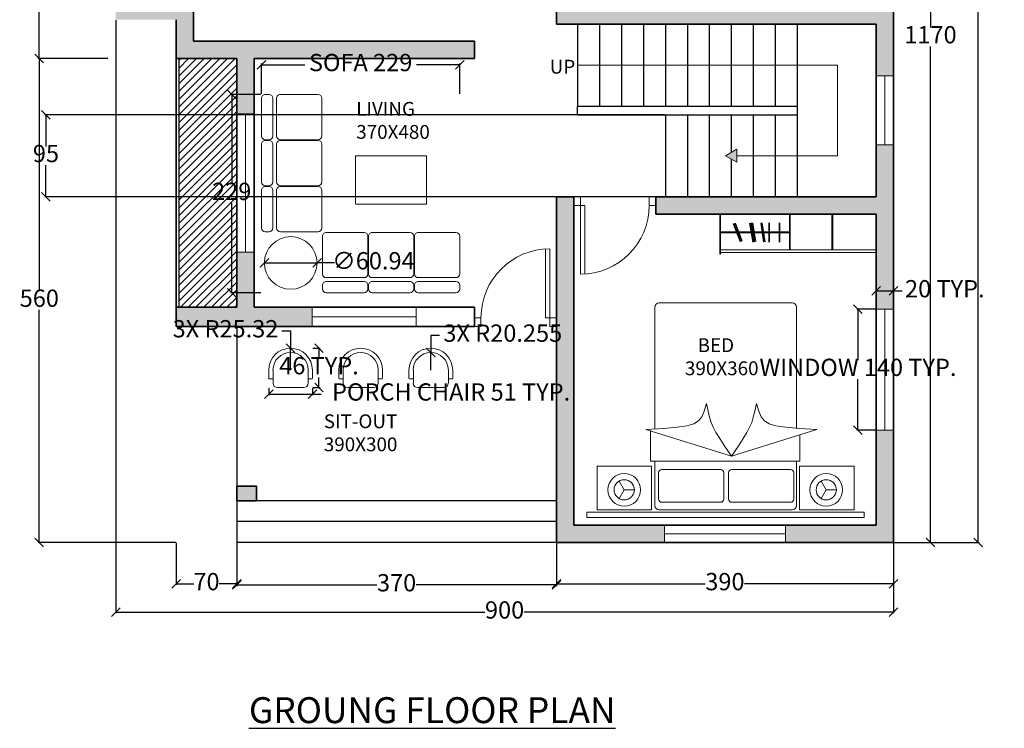
# Model space of a CAD drawing. Units: centimetres. Extents: x 2069 to 3209, y 376 to 1989.
# Tile 1 of 3: x 2069 to 3209, y 376 to 1196. Entities that reach past the tile are written whole.
import ezdxf

# ---------------------------------------------------------------- set-up
doc = ezdxf.new("R2010")
doc.units = ezdxf.units.CM
for name, color, linetype, lineweight in [('A-ANNO-DIMS', 2, 'Continuous', 18), ('A-ANNO-SYMB', 7, 'Continuous', 18), ('A-ANNO-TEXT', 7, 'Continuous', 25), ('A-AREA-IDEN', 7, 'Continuous', 25), ('A-COLS', 7, 'Continuous', 35), ('A-DOOR', 3, 'Continuous', 18), ('A-FLOR', 7, 'Continuous', 25), ('A-FLOR-CASE', 8, 'Continuous', 18), ('A-FLOR-PATT', 8, 'Continuous', 13), ('A-FLOR-STRS', 7, 'Continuous', 25), ('A-FURN', 8, 'Continuous', 18), ('A-GLAZ', 4, 'Continuous', 18), ('A-WALL', 7, 'Continuous', 35), ('A-WALL-PATT', 252, 'Continuous', 13)]:
    doc.layers.add(name, color=color, linetype=linetype, lineweight=lineweight)
doc.styles.get("Standard").update_dxf_attribs({"font": 'arial.ttf'})
doc.dimstyles.new('ISO-25', dxfattribs={"dimtxt": 20, "dimasz": 10, "dimexe": 1.25, "dimexo": 0.625, "dimtad": 0, "dimtih": 1, "dimtoh": 1, "dimtxsty": 'Standard', "dimblk": 'OBLIQUE', "dimcen": 6, "dimadec": 0, "dimazin": 0, "dimtfac": 1, "dimtmove": 0, "dimatfit": 3, "dimldrblk": 'OBLIQUE', "dimfxl": 1, "dimarcsym": 0})

# ---------------------------------------------------------------- blocks, each defined once
blk = doc.blocks.new('CAMMAT')
for p, q in [((1.2731, 0), (-1.2731, 0)), ((1.2731, 0), (1.2731, -0.05)), ((-1.2731, 0), (-1.2731, -0.05)), ((1.2731, -0.05), (-1.2731, -0.05)), ((-1.18, -0.07), (-1.18, -0.47)), ((-1.18, -0.07), (-0.68, -0.07)), ((-0.68, -0.07), (-0.68, -0.47)), ((0.61, -0.07), (-0.61, -0.07)), ((0.68, -0.07), (0.68, -0.47)), ((0.68, -0.07), (1.18, -0.07)), ((1.18, -0.07), (1.18, -0.47)), ((-0.931, -0.2541), (-0.9775, -0.1737)), ((-0.65, -0.11), (-0.65, -0.5169)), ((-0.6152, -0.1695), (-0.6152, -0.4095)), ((-0.0465, -0.1395), (-0.5852, -0.1395)), ((-0.0165, -0.1695), (-0.0165, -0.4095)), ((0.0274, -0.1695), (0.0274, -0.4095)), ((0.5962, -0.1395), (0.0574, -0.1395)), ((0.6262, -0.1695), (0.6262, -0.4095)), ((0.65, -0.11), (0.65, -0.5169)), ((0.9242, -0.2541), (0.8777, -0.1737)), ((-0.931, -0.2541), (-0.9775, -0.3346)), ((-0.931, -0.2541), (-0.8381, -0.2541)), ((0.9242, -0.2541), (0.8777, -0.3346)), ((0.9242, -0.2541), (1.0171, -0.2541)), ((-0.0465, -0.4395), (-0.5852, -0.4395)), ((0.5962, -0.4395), (0.0574, -0.4395)), ((-1.18, -0.47), (-0.68, -0.47)), ((-0.6904, -0.5169), (-0.6904, -0.8)), ((-0.6904, -0.5169), (0.6826, -0.5169)), ((0.68, -0.47), (1.18, -0.47)), ((0.6826, -0.5169), (0.6826, -0.7603)), ((0.0535, -0.5623), (-0.7312, -0.8093)), ((0.0535, -0.5623), (0.8382, -0.8093)), ((-0.65, -0.8139), (-0.65, -1.93)), ((0.65, -0.8204), (0.65, -1.93)), ((0.61, -1.97), (-0.61, -1.97))]:
    blk.add_line(p, q)
for points in [[(-0.1761, -1.0476), (-0.161, -0.9772), (-0.1474, -0.921), (-0.1326, -0.8732), (-0.1139, -0.8282), (-0.0886, -0.7803), (-0.0541, -0.7238), (-0.0076, -0.653), (0.0535, -0.5623)], [(0.2832, -1.0476), (0.2681, -0.9772), (0.2545, -0.921), (0.2396, -0.8732), (0.2209, -0.8282), (0.1957, -0.7803), (0.1611, -0.7238), (0.1147, -0.653), (0.0535, -0.5623)], [(-0.7312, -0.8093), (-0.5683, -0.8185), (-0.4451, -0.828), (-0.3552, -0.8406), (-0.2919, -0.8591), (-0.2489, -0.8862), (-0.2196, -0.9248), (-0.1975, -0.9777), (-0.1761, -1.0476)], [(0.8382, -0.8093), (0.6753, -0.8185), (0.5522, -0.828), (0.4622, -0.8406), (0.399, -0.8591), (0.356, -0.8862), (0.3267, -0.9248), (0.3046, -0.9777), (0.2832, -1.0476)]]:
    blk.add_lwpolyline(points)
for centre, radius in [((-0.931, -0.2541), 0.15), ((-0.931, -0.2541), 0.0929), ((0.9242, -0.2541), 0.15), ((0.9242, -0.2541), 0.0929)]:
    blk.add_circle(centre, radius)
for centre, radius, start, end in [((-0.61, -0.11), 0.04, 90, 180), ((0.61, -0.11), 0.04, 0, 90), ((-0.5852, -0.1695), 0.03, 90, 180), ((-0.0465, -0.1695), 0.03, 360, 90), ((0.0574, -0.1695), 0.03, 90, 180), ((0.5962, -0.1695), 0.03, 360, 90), ((-0.5852, -0.4095), 0.03, 180, 270), ((-0.0465, -0.4095), 0.03, 270, 360), ((0.0574, -0.4095), 0.03, 180, 270), ((0.5962, -0.4095), 0.03, 270, 360), ((-0.61, -1.93), 0.04, 180, 270), ((0.61, -1.93), 0.04, 270, 360)]:
    blk.add_arc(centre, radius, start, end)
blk = doc.blocks.new('A$C753D6792')
at = {"linetype": 'ByBlock'}
for p, q in [((50, 2630), (550, 2630)), ((660, 2630), (1160, 2630)), ((1270, 2630), (1770, 2630)), ((0, 2530), (0, 2580)), ((600, 2580), (600, 2530)), ((610, 2530), (610, 2580)), ((1210, 2580), (1210, 2530)), ((1220, 2530), (1220, 2580)), ((1820, 2580), (1820, 2530)), ((0, 1880), (0, 2380)), ((550, 2480), (50, 2480)), ((550, 2430), (50, 2430)), ((600, 2380), (600, 1880)), ((610, 1880), (610, 2380)), ((1160, 2480), (660, 2480)), ((1160, 2430), (660, 2430)), ((1210, 2380), (1210, 1880)), ((1220, 1880), (1220, 2380)), ((1770, 2480), (1270, 2480)), ((1770, 2430), (1270, 2430)), ((1820, 1880), (1820, 2380)), ((50, 1830), (427, 1830)), ((387, 1830), (550, 1830)), ((660, 1830), (1037, 1830)), ((997, 1830), (1160, 1830)), ((1270, 1830), (1647, 1830)), ((1607, 1830), (1770, 1830)), ((1830, 1770), (1830, 1393)), ((1880, 1820), (2380, 1820)), ((2430, 1270), (2430, 1770)), ((2480, 1270), (2480, 1770)), ((2530, 1820), (2580, 1820)), ((2630, 1770), (2630, 1270)), ((442, 815), (442, 1455)), ((442, 1455), (1372, 1455)), ((1382, 1455), (1382, 815)), ((1830, 1433), (1830, 1270)), ((2380, 1220), (1880, 1220)), ((1880, 1210), (2380, 1210)), ((2580, 1220), (2530, 1220)), ((2530, 1210), (2580, 1210)), ((1830, 1160), (1830, 783)), ((2430, 660), (2430, 1160)), ((2480, 660), (2480, 1160)), ((2630, 1160), (2630, 660)), ((1382, 815), (442, 815)), ((1830, 823), (1830, 660)), ((1830, 550), (1830, 173)), ((2380, 610), (1880, 610)), ((1880, 600), (2380, 600)), ((2430, 50), (2430, 550)), ((2480, 50), (2480, 550)), ((2580, 610), (2530, 610)), ((2530, 600), (2580, 600)), ((2630, 550), (2630, 50)), ((1830, 213), (1830, 50)), ((2380, 0), (1880, 0)), ((2580, 0), (2530, 0))]:
    blk.add_line(p, q, dxfattribs=at)
blk.add_circle((2242, 2235), 349, dxfattribs=at)
for centre, start, end in [((50, 2580), 90, 180), ((550, 2580), 0, 90), ((550, 2580), 0, 90), ((660, 2580), 90, 180), ((1160, 2580), 0, 90), ((1160, 2580), 0, 90), ((1270, 2580), 90, 180), ((1770, 2580), 0, 90), ((1770, 2580), 0, 90), ((50, 2530), 180, 270), ((550, 2530), 270, 0), ((550, 2530), 270, 0), ((660, 2530), 180, 270), ((1160, 2530), 270, 0), ((1160, 2530), 270, 0), ((1270, 2530), 180, 270), ((1770, 2530), 270, 0), ((1770, 2530), 270, 0), ((50, 2380), 90, 180), ((550, 2380), 0, 90), ((550, 2380), 0, 90), ((660, 2380), 90, 180), ((1160, 2380), 0, 90), ((1160, 2380), 0, 90), ((1270, 2380), 90, 180), ((1770, 2380), 0, 90), ((1770, 2380), 0, 90), ((50, 1880), 180, 270), ((550, 1880), 270, 0), ((660, 1880), 180, 270), ((1160, 1880), 270, 0), ((1270, 1880), 180, 270), ((1770, 1880), 270, 0), ((1880, 1770), 90, 180), ((2380, 1770), 0, 90), ((2530, 1770), 90, 180), ((2580, 1770), 0, 90), ((1880, 1270), 180, 270), ((1880, 1160), 90, 180), ((2380, 1270), 270, 0), ((2380, 1270), 270, 0), ((2380, 1160), 0, 90), ((2530, 1270), 180, 270), ((2530, 1270), 180, 270), ((2530, 1160), 90, 180), ((2580, 1270), 270, 0), ((2580, 1270), 270, 0), ((2580, 1160), 0, 90), ((1880, 660), 180, 270), ((2380, 660), 270, 0), ((2380, 660), 270, 0), ((2530, 660), 180, 270), ((2530, 660), 180, 270), ((2580, 660), 270, 0), ((2580, 660), 270, 0), ((1880, 550), 90, 180), ((2380, 550), 0, 90), ((2530, 550), 90, 180), ((2580, 550), 0, 90), ((1880, 50), 180, 270), ((2380, 50), 270, 0), ((2380, 50), 270, 0), ((2530, 50), 180, 270), ((2530, 50), 180, 270), ((2580, 50), 270, 0), ((2580, 50), 270, 0)]:
    blk.add_arc(centre, 50, start, end, dxfattribs=at)
blk = doc.blocks.new('_Oblique')
at = {"color": 0, "linetype": 'ByBlock', "lineweight": -2}
blk.add_line((-0.5, -0.5), (0.5, 0.5), dxfattribs=at)
blk = doc.blocks.new('*D16')
at = {"layer": 'A-ANNO-DIMS', "color": 0, "lineweight": -2, "transparency": 16777216}
for p, q in [((3081, 1761.2), (3124.6, 1761.2)), ((3123.3, 1761.2), (3123.3, 1187)), ((3123.3, 591.2), (3123.3, 1165.3)), ((3081, 591.2), (3124.6, 591.2))]:
    blk.add_line(p, q, dxfattribs=at)
at = {"layer": 'Defpoints', "color": 0, "transparency": 16777216}
for p in [(3080.4, 1761.2), (3080.4, 591.2), (3123.3, 591.2)]:
    blk.add_point(p, dxfattribs=at)
at = {"layer": 'A-ANNO-DIMS', "color": 0, "lineweight": -2, "transparency": 16777216, "xscale": 10, "yscale": 10, "zscale": 10}
for p, rotation in [((3123.3, 1761.2), 90), ((3123.3, 591.2), 270)]:
    blk.add_blockref('_Oblique', p, dxfattribs=dict(at, rotation=rotation))
at = {"layer": 'A-ANNO-DIMS', "color": 0, "transparency": 16777216, "insert": (3123.3, 1176.2), "char_height": 20, "attachment_point": 5}
blk.add_mtext('1170', dxfattribs=at)
blk = doc.blocks.new('*D17')
at = {"layer": 'A-ANNO-DIMS', "color": 0, "lineweight": -2, "transparency": 16777216}
for p, q in [((2690.4, 590.6), (2690.4, 541.9)), ((3080.4, 590.6), (3080.4, 541.9)), ((2690.4, 543.2), (2862.7, 543.2)), ((3080.4, 543.2), (2908.1, 543.2))]:
    blk.add_line(p, q, dxfattribs=at)
at = {"layer": 'Defpoints', "color": 0, "transparency": 16777216}
for p in [(2690.4, 591.2), (3080.4, 591.2), (2690.4, 543.2)]:
    blk.add_point(p, dxfattribs=at)
at = {"layer": 'A-ANNO-DIMS', "color": 0, "lineweight": -2, "transparency": 16777216, "xscale": 10, "yscale": 10, "zscale": 10, "rotation": 180}
blk.add_blockref('_Oblique', (2690.4, 543.2), dxfattribs=at)
at = {"layer": 'A-ANNO-DIMS', "color": 0, "lineweight": -2, "transparency": 16777216, "xscale": 10, "yscale": 10, "zscale": 10}
blk.add_blockref('_Oblique', (3080.4, 543.2), dxfattribs=at)
at = {"layer": 'A-ANNO-DIMS', "color": 0, "transparency": 16777216, "insert": (2885.4, 543.2), "char_height": 20, "attachment_point": 5}
blk.add_mtext('390', dxfattribs=at)
blk = doc.blocks.new('*D18')
at = {"layer": 'A-ANNO-DIMS', "color": 0, "lineweight": -2, "transparency": 16777216}
for p, q in [((2320.4, 590.6), (2320.4, 540.7)), ((2690.4, 590.6), (2690.4, 540.7)), ((2320.4, 541.9), (2482.7, 541.9)), ((2690.4, 541.9), (2528.1, 541.9))]:
    blk.add_line(p, q, dxfattribs=at)
at = {"layer": 'Defpoints', "color": 0, "transparency": 16777216}
for p in [(2320.4, 591.2), (2690.4, 591.2), (2320.4, 541.9)]:
    blk.add_point(p, dxfattribs=at)
at = {"layer": 'A-ANNO-DIMS', "color": 0, "lineweight": -2, "transparency": 16777216, "xscale": 10, "yscale": 10, "zscale": 10, "rotation": 180}
blk.add_blockref('_Oblique', (2320.4, 541.9), dxfattribs=at)
at = {"layer": 'A-ANNO-DIMS', "color": 0, "lineweight": -2, "transparency": 16777216, "xscale": 10, "yscale": 10, "zscale": 10}
blk.add_blockref('_Oblique', (2690.4, 541.9), dxfattribs=at)
at = {"layer": 'A-ANNO-DIMS', "color": 0, "transparency": 16777216, "insert": (2505.4, 541.9), "char_height": 20, "attachment_point": 5}
blk.add_mtext('370', dxfattribs=at)
blk = doc.blocks.new('*D19')
at = {"layer": 'A-ANNO-DIMS', "color": 0, "lineweight": -2, "transparency": 16777216}
for p, q in [((2250.4, 590.6), (2250.4, 541.9)), ((2320.4, 590.6), (2320.4, 541.9)), ((2250.4, 543.2), (2270.6, 543.2)), ((2320.4, 543.2), (2300.2, 543.2))]:
    blk.add_line(p, q, dxfattribs=at)
at = {"layer": 'Defpoints', "color": 0, "transparency": 16777216}
for p in [(2250.4, 591.2), (2320.4, 591.2), (2320.4, 543.2)]:
    blk.add_point(p, dxfattribs=at)
at = {"layer": 'A-ANNO-DIMS', "color": 0, "lineweight": -2, "transparency": 16777216, "xscale": 10, "yscale": 10, "zscale": 10, "rotation": 180}
blk.add_blockref('_Oblique', (2250.4, 543.2), dxfattribs=at)
at = {"layer": 'A-ANNO-DIMS', "color": 0, "lineweight": -2, "transparency": 16777216, "xscale": 10, "yscale": 10, "zscale": 10}
blk.add_blockref('_Oblique', (2320.4, 543.2), dxfattribs=at)
at = {"layer": 'A-ANNO-DIMS', "color": 0, "transparency": 16777216, "insert": (2285.4, 543.2), "char_height": 20, "attachment_point": 5}
blk.add_mtext('70', dxfattribs=at)
blk = doc.blocks.new('*D21')
at = {"layer": 'A-ANNO-DIMS', "color": 0, "lineweight": -2, "transparency": 16777216}
for p, q in [((2170.2, 1521.2), (2090.7, 1521.2)), ((2091.9, 1521.2), (2091.9, 1347)), ((2091.9, 1151.2), (2091.9, 1325.3)), ((2171.1, 1151.2), (2090.7, 1151.2))]:
    blk.add_line(p, q, dxfattribs=at)
at = {"layer": 'Defpoints', "color": 0, "transparency": 16777216}
for p in [(2170.8, 1521.2), (2091.9, 1151.2), (2171.7, 1151.2)]:
    blk.add_point(p, dxfattribs=at)
at = {"layer": 'A-ANNO-DIMS', "color": 0, "lineweight": -2, "transparency": 16777216, "xscale": 10, "yscale": 10, "zscale": 10}
for p, rotation in [((2091.9, 1521.2), 90), ((2091.9, 1151.2), 270)]:
    blk.add_blockref('_Oblique', p, dxfattribs=dict(at, rotation=rotation))
at = {"layer": 'A-ANNO-DIMS', "color": 0, "transparency": 16777216, "insert": (2091.9, 1336.2), "char_height": 20, "attachment_point": 5}
blk.add_mtext('370', dxfattribs=at)
blk = doc.blocks.new('*D22')
at = {"layer": 'A-ANNO-DIMS', "color": 0, "lineweight": -2, "transparency": 16777216}
for p, q in [((2169.6, 1151.2), (2090.7, 1151.2)), ((2091.9, 1151.2), (2091.9, 882)), ((2091.9, 591.2), (2091.9, 860.3)), ((2249.8, 591.2), (2090.7, 591.2))]:
    blk.add_line(p, q, dxfattribs=at)
at = {"layer": 'Defpoints', "color": 0, "transparency": 16777216}
for p in [(2170.2, 1151.2), (2091.9, 591.2), (2250.4, 591.2)]:
    blk.add_point(p, dxfattribs=at)
at = {"layer": 'A-ANNO-DIMS', "color": 0, "lineweight": -2, "transparency": 16777216, "xscale": 10, "yscale": 10, "zscale": 10}
for p, rotation in [((2091.9, 1151.2), 90), ((2091.9, 591.2), 270)]:
    blk.add_blockref('_Oblique', p, dxfattribs=dict(at, rotation=rotation))
at = {"layer": 'A-ANNO-DIMS', "color": 0, "transparency": 16777216, "insert": (2091.9, 871.2), "char_height": 20, "attachment_point": 5}
blk.add_mtext('560', dxfattribs=at)
blk = doc.blocks.new('CHAIR-SITOUT')
for p, q in [((0, 11.1), (0, 20.3)), ((5.1, 20.3), (5.1, 5.1)), ((45.6, 5.1), (45.6, 20.3)), ((50.6, 11.1), (50.6, 20.3)), ((1, 10.1), (5.1, 10.1)), ((10.1, 0), (40.5, 0)), ((45.6, 10.1), (49.6, 10.1))]:
    blk.add_line(p, q)
for centre, radius, start, end in [((25.3, 20.3), 25.3, 0, 180), ((25.3, 20.3), 20.3, 0.0001, 179.9999), ((1, 11.1), 1.01, 180, 270), ((10.1, 5.1), 5.06, 180, 270), ((40.5, 5.1), 5.06, 270, 0), ((49.6, 11.1), 1.01, 270, 0)]:
    blk.add_arc(centre, radius, start, end)
blk = doc.blocks.new('WIN-1400')
for p, q in [((0, 140), (20, 140)), ((10, 0), (10, 140)), ((0, 0), (20, 0))]:
    blk.add_line(p, q)
blk = doc.blocks.new('DOOR-SINGLE-950')
for p, q in [((82.3, 89.4), (82.3, 10)), ((87.3, 89.6), (87.3, 10)), ((0, 10), (7.7, 10)), ((7.7, 10), (7.7, 0)), ((82.3, 10), (87.3, 10)), ((95, 10), (87.3, 10)), ((87.3, 10), (87.3, 0)), ((7.7, 0), (0, 0)), ((87.3, 0), (95, 0))]:
    blk.add_line(p, q)
blk.add_arc((87.3, 10), 79.6, 90, 180)
blk = doc.blocks.new('*D32')
at = {"layer": 'A-ANNO-DIMS', "color": 0, "lineweight": -2, "transparency": 16777216}
for p, q in [((2357.4, 769.7), (2357.4, 761.4)), ((2408, 769.7), (2408, 761.4)), ((2357.4, 762.7), (2408, 762.7)), ((2408, 762.7), (2418, 762.7))]:
    blk.add_line(p, q, dxfattribs=at)
at = {"layer": 'Defpoints', "color": 0, "transparency": 16777216}
for p in [(2357.4, 770.3), (2408, 770.3), (2408, 762.7)]:
    blk.add_point(p, dxfattribs=at)
at = {"layer": 'A-ANNO-DIMS', "color": 0, "lineweight": -2, "transparency": 16777216, "xscale": 10, "yscale": 10, "zscale": 10, "rotation": 180}
blk.add_blockref('_Oblique', (2357.4, 762.7), dxfattribs=at)
at = {"layer": 'A-ANNO-DIMS', "color": 0, "lineweight": -2, "transparency": 16777216, "xscale": 10, "yscale": 10, "zscale": 10}
blk.add_blockref('_Oblique', (2408, 762.7), dxfattribs=at)
at = {"layer": 'A-ANNO-DIMS', "color": 0, "transparency": 16777216, "insert": (2568.5, 762.7), "char_height": 20, "attachment_point": 5}
blk.add_mtext('PORCH CHAIR 51 TYP.', dxfattribs=at)
blk = doc.blocks.new('*D33')
at = {"layer": 'A-ANNO-DIMS', "color": 0, "lineweight": -2, "transparency": 16777216}
for p, q in [((2408.6, 815.9), (2416.8, 815.9)), ((2415.6, 815.9), (2415.6, 803.9)), ((2415.6, 770.3), (2415.6, 782.2)), ((2408.6, 770.3), (2416.8, 770.3))]:
    blk.add_line(p, q, dxfattribs=at)
at = {"layer": 'Defpoints', "color": 0, "transparency": 16777216}
for p in [(2408, 815.9), (2415.6, 815.9), (2408, 770.3)]:
    blk.add_point(p, dxfattribs=at)
at = {"layer": 'A-ANNO-DIMS', "color": 0, "lineweight": -2, "transparency": 16777216, "xscale": 10, "yscale": 10, "zscale": 10}
for p, rotation in [((2415.6, 815.9), 90), ((2415.6, 770.3), 270)]:
    blk.add_blockref('_Oblique', p, dxfattribs=dict(at, rotation=rotation))
at = {"layer": 'A-ANNO-DIMS', "color": 0, "transparency": 16777216, "insert": (2415.6, 793.1), "char_height": 20, "attachment_point": 5}
blk.add_mtext('46 TYP.', dxfattribs=at)
blk = doc.blocks.new('*D34')
at = {"layer": 'A-ANNO-DIMS', "color": 0, "lineweight": -2, "transparency": 16777216}
for p, q in [((3059.8, 861.2), (3038.1, 861.2)), ((3039.4, 861.2), (3039.4, 802.2)), ((3039.4, 721.2), (3039.4, 780.2)), ((3059.8, 721.2), (3038.1, 721.2))]:
    blk.add_line(p, q, dxfattribs=at)
at = {"layer": 'Defpoints', "color": 0, "transparency": 16777216}
for p in [(3039.4, 861.2), (3060.4, 861.2), (3060.4, 721.2)]:
    blk.add_point(p, dxfattribs=at)
at = {"layer": 'A-ANNO-DIMS', "color": 0, "lineweight": -2, "transparency": 16777216, "xscale": 10, "yscale": 10, "zscale": 10}
for p, rotation in [((3039.4, 861.2), 90), ((3039.4, 721.2), 270)]:
    blk.add_blockref('_Oblique', p, dxfattribs=dict(at, rotation=rotation))
at = {"layer": 'A-ANNO-DIMS', "color": 0, "transparency": 16777216, "insert": (3039.4, 791.2), "char_height": 20, "attachment_point": 5}
blk.add_mtext('WINDOW 140 TYP.', dxfattribs=at)
blk = doc.blocks.new('*D35')
at = {"layer": 'A-ANNO-DIMS', "color": 0, "lineweight": -2, "transparency": 16777216}
for p, q in [((3060.4, 861.8), (3060.4, 883.4)), ((3060.4, 882.2), (3080.4, 882.2)), ((3080.4, 861.8), (3080.4, 883.4)), ((3080.4, 882.2), (3090.4, 882.2))]:
    blk.add_line(p, q, dxfattribs=at)
at = {"layer": 'Defpoints', "color": 0, "transparency": 16777216}
for p in [(3080.4, 882.2), (3060.4, 861.2), (3080.4, 861.2)]:
    blk.add_point(p, dxfattribs=at)
at = {"layer": 'A-ANNO-DIMS', "color": 0, "lineweight": -2, "transparency": 16777216, "xscale": 10, "yscale": 10, "zscale": 10, "rotation": 180}
blk.add_blockref('_Oblique', (3060.4, 882.2), dxfattribs=at)
at = {"layer": 'A-ANNO-DIMS', "color": 0, "lineweight": -2, "transparency": 16777216, "xscale": 10, "yscale": 10, "zscale": 10}
blk.add_blockref('_Oblique', (3080.4, 882.2), dxfattribs=at)
at = {"layer": 'A-ANNO-DIMS', "color": 0, "transparency": 16777216, "insert": (3139.9, 882.2), "char_height": 20, "attachment_point": 5}
blk.add_mtext('20 TYP.', dxfattribs=at)
blk = doc.blocks.new('*D44')
at = {"layer": 'A-ANNO-DIMS', "color": 0, "lineweight": -2, "transparency": 16777216}
for p, q in [((2349.1, 1110.2), (2349.1, 1145.3)), ((2349.1, 1144), (2399.2, 1144)), ((2578.5, 1144), (2528.4, 1144)), ((2578.5, 1110.2), (2578.5, 1145.3))]:
    blk.add_line(p, q, dxfattribs=at)
at = {"layer": 'Defpoints', "color": 0, "transparency": 16777216}
for p in [(2349.1, 1144), (2349.1, 1109.6), (2578.5, 1109.6)]:
    blk.add_point(p, dxfattribs=at)
at = {"layer": 'A-ANNO-DIMS', "color": 0, "lineweight": -2, "transparency": 16777216, "xscale": 10, "yscale": 10, "zscale": 10, "rotation": 180}
blk.add_blockref('_Oblique', (2349.1, 1144), dxfattribs=at)
at = {"layer": 'A-ANNO-DIMS', "color": 0, "lineweight": -2, "transparency": 16777216, "xscale": 10, "yscale": 10, "zscale": 10}
blk.add_blockref('_Oblique', (2578.5, 1144), dxfattribs=at)
at = {"layer": 'A-ANNO-DIMS', "color": 0, "transparency": 16777216, "insert": (2463.8, 1144), "char_height": 20, "attachment_point": 5}
blk.add_mtext('SOFA 229', dxfattribs=at)
blk = doc.blocks.new('*D45')
at = {"layer": 'A-ANNO-DIMS', "color": 0, "lineweight": -2, "transparency": 16777216}
for p, q in [((2348.4, 1109.6), (2313.4, 1109.6)), ((2314.6, 1109.6), (2314.6, 1005.7)), ((2314.6, 880.1), (2314.6, 984)), ((2348.4, 880.1), (2313.4, 880.1))]:
    blk.add_line(p, q, dxfattribs=at)
at = {"layer": 'Defpoints', "color": 0, "transparency": 16777216}
for p in [(2349.1, 1109.6), (2314.6, 880.1), (2349.1, 880.1)]:
    blk.add_point(p, dxfattribs=at)
at = {"layer": 'A-ANNO-DIMS', "color": 0, "lineweight": -2, "transparency": 16777216, "xscale": 10, "yscale": 10, "zscale": 10}
for p, rotation in [((2314.6, 1109.6), 90), ((2314.6, 880.1), 270)]:
    blk.add_blockref('_Oblique', p, dxfattribs=dict(at, rotation=rotation))
at = {"layer": 'A-ANNO-DIMS', "color": 0, "transparency": 16777216, "insert": (2314.6, 994.9), "char_height": 20, "attachment_point": 5}
blk.add_mtext('229', dxfattribs=at)
blk = doc.blocks.new('*D46')
at = {"layer": 'A-ANNO-DIMS', "color": 0, "lineweight": -2, "transparency": 16777216}
for p, q in [((2180.4, 1195.6), (2180.4, 509.1)), ((3080.4, 590.6), (3080.4, 509.1)), ((2180.4, 510.4), (2607.7, 510.4)), ((3080.4, 510.4), (2653.1, 510.4))]:
    blk.add_line(p, q, dxfattribs=at)
at = {"layer": 'Defpoints', "color": 0, "transparency": 16777216}
for p in [(2180.4, 1196.2), (3080.4, 591.2), (3080.4, 510.4)]:
    blk.add_point(p, dxfattribs=at)
at = {"layer": 'A-ANNO-DIMS', "color": 0, "lineweight": -2, "transparency": 16777216, "xscale": 10, "yscale": 10, "zscale": 10, "rotation": 180}
blk.add_blockref('_Oblique', (2180.4, 510.4), dxfattribs=at)
at = {"layer": 'A-ANNO-DIMS', "color": 0, "lineweight": -2, "transparency": 16777216, "xscale": 10, "yscale": 10, "zscale": 10}
blk.add_blockref('_Oblique', (3080.4, 510.4), dxfattribs=at)
at = {"layer": 'A-ANNO-DIMS', "color": 0, "transparency": 16777216, "insert": (2630.4, 510.4), "char_height": 20, "attachment_point": 5}
blk.add_mtext('900', dxfattribs=at)
blk = doc.blocks.new('*D47')
at = {"layer": 'A-ANNO-DIMS', "color": 0, "lineweight": -2, "transparency": 16777216}
for p, q in [((2711, 1941.2), (3179.7, 1941.2)), ((3178.5, 1941.2), (3178.5, 1277)), ((3178.5, 591.2), (3178.5, 1255.3)), ((3081, 591.2), (3179.7, 591.2))]:
    blk.add_line(p, q, dxfattribs=at)
at = {"layer": 'Defpoints', "color": 0, "transparency": 16777216}
for p in [(2710.4, 1941.2), (3080.4, 591.2), (3178.5, 591.2)]:
    blk.add_point(p, dxfattribs=at)
at = {"layer": 'A-ANNO-DIMS', "color": 0, "lineweight": -2, "transparency": 16777216, "xscale": 10, "yscale": 10, "zscale": 10}
for p, rotation in [((3178.5, 1941.2), 90), ((3178.5, 591.2), 270)]:
    blk.add_blockref('_Oblique', p, dxfattribs=dict(at, rotation=rotation))
at = {"layer": 'A-ANNO-DIMS', "color": 0, "transparency": 16777216, "insert": (3178.5, 1266.2), "char_height": 20, "attachment_point": 5}
blk.add_mtext('1350', dxfattribs=at)
blk = doc.blocks.new('*D48')
at = {"layer": 'A-ANNO-DIMS', "color": 0, "lineweight": -2, "transparency": 16777216}
for p, q in [((2815.9, 1086.2), (2098.3, 1086.2)), ((2099.6, 1086.2), (2099.6, 1049.5)), ((2099.6, 991.2), (2099.6, 1027.8)), ((2815.9, 991.2), (2098.3, 991.2))]:
    blk.add_line(p, q, dxfattribs=at)
at = {"layer": 'Defpoints', "color": 0, "transparency": 16777216}
for p in [(2099.6, 1086.2), (2816.5, 1086.2), (2816.5, 991.2)]:
    blk.add_point(p, dxfattribs=at)
at = {"layer": 'A-ANNO-DIMS', "color": 0, "lineweight": -2, "transparency": 16777216, "xscale": 10, "yscale": 10, "zscale": 10}
for p, rotation in [((2099.6, 1086.2), 90), ((2099.6, 991.2), 270)]:
    blk.add_blockref('_Oblique', p, dxfattribs=dict(at, rotation=rotation))
at = {"layer": 'A-ANNO-DIMS', "color": 0, "transparency": 16777216, "insert": (2099.6, 1038.7), "char_height": 20, "attachment_point": 5}
blk.add_mtext('95', dxfattribs=at)
blk = doc.blocks.new('*D49')
at = {"layer": 'A-ANNO-DIMS', "color": 0, "lineweight": -2, "transparency": 16777216}
for p in [(2352.4, 914.6), (2433.4, 914.6)]:
    blk.add_line(p, (2413.4, 914.6), dxfattribs=at)
at = {"layer": 'Defpoints', "color": 0, "transparency": 16777216}
for p in [(2352.4, 914.6), (2413.4, 914.6)]:
    blk.add_point(p, dxfattribs=at)
at = {"layer": 'A-ANNO-DIMS', "color": 0, "lineweight": -2, "transparency": 16777216, "xscale": 10, "yscale": 10, "zscale": 10}
for p, rotation in [((2352.4, 914.6), 0.0003591282010973), ((2413.4, 914.6), 180.0003591282011)]:
    blk.add_blockref('_Oblique', p, dxfattribs=dict(at, rotation=rotation))
at = {"layer": 'A-ANNO-DIMS', "color": 0, "transparency": 16777216, "insert": (2478.6, 914.6), "char_height": 20, "attachment_point": 5}
blk.add_mtext('∅60.94', dxfattribs=at)
blk = doc.blocks.new('*D53')
at = {"layer": 'A-ANNO-DIMS', "color": 0, "lineweight": -2, "transparency": 16777216}
for p, q in [((2372.7, 835.9), (2382.7, 835.9)), ((2382.7, 835.9), (2382.7, 815.9)), ((2382.7, 790.5), (2382.7, 815.9))]:
    blk.add_line(p, q, dxfattribs=at)
at = {"layer": 'Defpoints', "color": 0, "transparency": 16777216}
for p in [(2382.7, 815.9), (2382.7, 790.5)]:
    blk.add_point(p, dxfattribs=at)
at = {"layer": 'A-ANNO-DIMS', "color": 0, "lineweight": -2, "transparency": 16777216, "xscale": 10, "yscale": 10, "zscale": 10, "rotation": 270.0002308247618}
blk.add_blockref('_Oblique', (2382.7, 815.9), dxfattribs=at)
at = {"layer": 'A-ANNO-DIMS', "color": 0, "transparency": 16777216, "insert": (2307.4, 835.9), "char_height": 20, "attachment_point": 5}
blk.add_mtext('3X R25.32', dxfattribs=at)
blk = doc.blocks.new('*D54')
at = {"layer": 'A-ANNO-DIMS', "color": 0, "lineweight": -2, "transparency": 16777216}
for p, q in [((2555, 830.8), (2545, 830.8)), ((2545, 830.8), (2545, 810.8)), ((2545, 790.5), (2545, 810.8))]:
    blk.add_line(p, q, dxfattribs=at)
at = {"layer": 'Defpoints', "color": 0, "transparency": 16777216}
for p in [(2545, 810.8), (2545, 790.5)]:
    blk.add_point(p, dxfattribs=at)
at = {"layer": 'A-ANNO-DIMS', "color": 0, "lineweight": -2, "transparency": 16777216, "xscale": 10, "yscale": 10, "zscale": 10, "rotation": 269.9991683519763}
blk.add_blockref('_Oblique', (2545, 810.8), dxfattribs=at)
at = {"layer": 'A-ANNO-DIMS', "color": 0, "transparency": 16777216, "insert": (2628.3, 830.8), "char_height": 20, "attachment_point": 5}
blk.add_mtext('3X R20.255', dxfattribs=at)

msp = doc.modelspace()

# ---------------------------------------------------------------- hatches: boundary and pattern name
at = {"layer": 'A-ANNO-SYMB'}
h = msp.add_hatch(color=256, dxfattribs=at)
h.dxf.hatch_style = 1
h.paths.add_polyline_path([(2899.1177, 1046.245), (2886.018, 1038.6819), (2899.1177, 1031.1188)])
at = {"layer": 'A-FLOR-PATT'}
h = msp.add_hatch(dxfattribs=at)
h.set_pattern_fill('ANSI31', color=256, scale=2)
h.paths.add_polyline_path([(2320.3865, 1151.1819), (2253.3865, 1151.1819), (2253.3865, 863.2574), (2320.3865, 863.2574)])
at = {"layer": 'A-WALL-PATT'}
h = msp.add_hatch(color=256, dxfattribs=at)
h.dxf.hatch_style = 1
h.paths.add_polyline_path([(2498.1872, 1921.1819), (2498.1872, 1941.1819), (2320.3865, 1941.1819), (2320.3865, 1616.1819), (2340.3865, 1616.1819), (2340.3865, 1921.1819)])
h.paths.add_polyline_path([(2690.3865, 1921.1819), (2690.3865, 1456.1819), (2710.3865, 1456.1819), (2710.3865, 1741.1819), (2742.2674, 1741.1819), (2742.2674, 1761.1819), (2710.3865, 1761.1819), (2710.3865, 1941.1819), (2618.1872, 1941.1819), (2618.1872, 1921.1819)])
h.paths.add_polyline_path([(2802.2674, 1761.1819), (2802.2674, 1741.1819), (2971.3879, 1741.1819), (2971.3879, 1761.1819)])
h.paths.add_polyline_path([(3080.3865, 1761.1819), (3031.3879, 1761.1819), (3031.3879, 1741.1819), (3060.3865, 1741.1819), (3060.3865, 1621.1819), (3080.3865, 1621.1819)])
h.paths.add_polyline_path([(3060.3865, 1361.1819), (2906.9077, 1361.1819), (2906.9077, 1341.1819), (3060.3865, 1341.1819), (3060.3865, 1296.1819), (3080.3865, 1296.1819), (3080.3865, 1481.1819), (3060.3865, 1481.1819)])
h.paths.add_polyline_path([(2799.9077, 1341.1819), (2799.9077, 1211.1819), (2690.3865, 1211.1819), (2690.3865, 1191.1819), (3060.3865, 1191.1819), (3060.3865, 1131.1819), (3080.3865, 1131.1819), (3080.3865, 1256.1819), (3060.3865, 1256.1819), (3060.3865, 1211.1819), (2821.9077, 1211.1819), (2821.9077, 1361.1819), (2690.3865, 1361.1819), (2690.3865, 1341.1819)])
h.paths.add_polyline_path([(3080.3865, 1051.1819), (3060.3865, 1051.1819), (3060.3865, 991.1819), (2805.3865, 991.1819), (2805.3865, 971.1819), (3060.3865, 971.1819), (3060.3865, 861.1819), (3080.3865, 861.1819)])
h.paths.add_polyline_path([(2690.3865, 591.1819), (2815.3865, 591.1819), (2815.3865, 611.1819), (2710.3865, 611.1819), (2710.3865, 991.1819), (2690.3865, 991.1819)])
h.paths.add_polyline_path([(2955.3865, 611.1819), (2955.3865, 591.1819), (3080.3865, 591.1819), (3080.3865, 721.1819), (3060.3865, 721.1819), (3060.3865, 611.1819)])
h.paths.add_polyline_path([(2320.3865, 656.2562), (2320.3865, 639.1819), (2343.1963, 639.1819), (2343.1963, 656.2562)])
h.paths.add_polyline_path([(2320.3865, 863.2574), (2250.3865, 863.2574), (2250.3865, 841.2574), (2407.8865, 841.2574), (2407.8865, 863.2574), (2340.3865, 863.2574), (2340.3865, 927.2197), (2320.3865, 927.2197)])
h.paths.add_polyline_path([(2320.3865, 1151.1819), (2320.3865, 1087.2197), (2340.3865, 1087.2197), (2340.3865, 1151.1819), (2595.3865, 1151.1819), (2595.3865, 1171.1819), (2270.3865, 1171.1819), (2270.3865, 1216.1819), (2180.3865, 1216.1819), (2180.3865, 1196.1819), (2250.3865, 1196.1819), (2250.3865, 1151.1819)])
h.paths.add_polyline_path([(2595.3865, 1501.1819), (2595.3865, 1521.1819), (2250.3865, 1521.1819), (2250.3865, 1476.1819), (2180.3865, 1476.1819), (2180.3865, 1456.1819), (2270.3865, 1456.1819), (2270.3865, 1501.1819)])

# ---------------------------------------------------------------- linework, layer by layer
at = {"layer": 'A-ANNO-SYMB'}
for p, q in [((2714.9465, 1143.6819), (3015.5322, 1143.6819)), ((3015.5322, 1143.6819), (3015.5322, 1038.6819)), ((2899.1177, 1038.6819), (3015.5322, 1038.6819))]:
    msp.add_line(p, q, dxfattribs=at)
msp.add_lwpolyline([(2886.018, 1038.6819), (2899.1177, 1031.1188), (2899.1177, 1046.245)], close=True, dxfattribs=at)
at = {"layer": 'A-COLS'}
msp.add_lwpolyline([(2320.3865, 639.1819), (2343.1963, 639.1819), (2343.1963, 656.2562), (2320.3865, 656.2562)], close=True, dxfattribs=at)
at = {"layer": 'A-FLOR'}
for p, q in [((2253.3865, 1151.1819), (2253.3865, 863.2574)), ((2320.3865, 841.2574), (2320.3865, 591.1819))]:
    msp.add_line(p, q, dxfattribs=at)
at = {"layer": 'A-FLOR-CASE'}
for p, q in [((2879.4739, 971.1819), (2879.4739, 924.8354)), ((2880.4739, 926.8354), (2880.4739, 971.1819)), ((2959.9749, 971.1819), (2959.9749, 929.8354)), ((2960.9749, 971.1819), (2960.9749, 929.8354)), ((3009.2394, 971.1819), (3009.2394, 929.8354)), ((3010.2394, 971.1819), (3010.2394, 929.8354)), ((2895.0566, 959.8608), (2902.9421, 939.1343)), ((2895.8986, 960.1812), (2903.7841, 939.4547)), ((2896.7407, 960.5016), (2904.6262, 939.7751)), ((2897.5828, 960.8219), (2905.4683, 940.0954)), ((2914.0161, 960.5964), (2917.5423, 938.7027)), ((2914.9056, 960.7396), (2918.4318, 938.8459)), ((2915.7951, 960.8829), (2919.3212, 938.9892)), ((2916.6845, 961.0262), (2920.2107, 939.1324)), ((2917.574, 961.1694), (2921.1002, 939.2757)), ((2926.8903, 960.7596), (2930.2488, 938.8396)), ((2927.7809, 960.8961), (2931.1394, 938.976)), ((2928.6714, 961.0325), (2932.0299, 939.1125)), ((2936.1816, 961.024), (2936.1816, 938.8481)), ((2937.0826, 961.024), (2937.0826, 938.8481)), ((2948.2377, 961.024), (2948.2377, 938.8481)), ((2949.1386, 961.024), (2949.1386, 938.8481)), ((2880.4739, 950.6216), (2959.9749, 950.6216)), ((2880.4739, 949.6216), (2959.9749, 949.6216)), ((2879.4739, 924.8354), (2880.4739, 924.8354)), ((2880.4739, 929.8354), (3060.3865, 929.8354)), ((2880.4739, 926.8354), (3060.3865, 926.8354)), ((2880.4739, 924.8354), (2880.4739, 926.8354)), ((2880.4739, 926.8354), (2880.4739, 926.8354))]:
    msp.add_line(p, q, dxfattribs=at)
at = {"layer": 'A-FLOR-STRS'}
for p, q in [((2714.9465, 1191.1819), (2714.9465, 1096.1819)), ((2740.3465, 1191.1819), (2740.3465, 1096.1819)), ((2765.7465, 1191.1819), (2765.7465, 1096.1819)), ((2791.1465, 1191.1819), (2791.1465, 1096.1819)), ((2816.5465, 1191.1819), (2816.5465, 1096.1819)), ((2841.9465, 1191.1819), (2841.9465, 1096.1819)), ((2867.3465, 1191.1819), (2867.3465, 1096.1819)), ((2892.7465, 1191.1819), (2892.7465, 1096.1819)), ((2918.1465, 1191.1819), (2918.1465, 1096.1819)), ((2943.5465, 1191.1819), (2943.5465, 1096.1819)), ((2968.9465, 1191.1819), (2968.9465, 991.1819)), ((2714.9465, 1096.1819), (2968.9465, 1096.1819)), ((2714.9465, 1086.1819), (2714.9465, 1096.1819)), ((2714.9465, 1086.1819), (2968.9465, 1086.1819)), ((2816.5465, 1086.1819), (2816.5465, 991.1819)), ((2841.9465, 1086.1819), (2841.9465, 991.1819)), ((2867.3465, 1086.1819), (2867.3465, 991.1819)), ((2892.7465, 1086.1819), (2892.7465, 1042.5666)), ((2918.1465, 1086.1819), (2918.1465, 991.1819)), ((2943.5465, 1086.1819), (2943.5465, 991.1819)), ((2892.7465, 1034.7972), (2892.7465, 991.1819)), ((2690.3865, 639.1819), (2320.3865, 639.1819)), ((2690.3865, 615.1819), (2320.3865, 615.1819)), ((2690.3865, 591.1819), (2320.3865, 591.1819))]:
    msp.add_line(p, q, dxfattribs=at)
at = {"layer": 'A-GLAZ'}
for p, q in [((3060.3865, 1131.1819), (3080.3865, 1131.1819)), ((3070.3865, 1051.1819), (3070.3865, 1131.1819)), ((2340.3865, 1087.2197), (2320.3865, 1087.2197)), ((2330.3865, 927.2197), (2330.3865, 1087.2197)), ((3060.3865, 1051.1819), (3080.3865, 1051.1819)), ((2340.3865, 927.2197), (2320.3865, 927.2197)), ((2407.8865, 863.2574), (2407.8865, 841.2574)), ((2527.8865, 863.2574), (2527.8865, 841.2574)), ((2527.8865, 852.2574), (2407.8865, 852.2574))]:
    msp.add_line(p, q, dxfattribs=at)
at = {"layer": 'A-WALL'}
for p, q in [((3080.3865, 1761.1819), (3080.3865, 591.1819)), ((2270.3865, 1501.1819), (2270.3865, 1171.1819)), ((2690.3865, 1211.1819), (2690.3865, 1191.1819)), ((2250.3865, 1196.1819), (2250.3865, 841.2574)), ((2690.3865, 1191.1819), (3060.3865, 1191.1819)), ((3060.3865, 1191.1819), (3060.3865, 991.1819)), ((2270.3865, 1171.1819), (2595.3865, 1171.1819)), ((2595.3865, 1171.1819), (2595.3865, 1151.1819)), ((2250.3865, 1151.1819), (2320.3865, 1151.1819)), ((2320.3865, 1151.1819), (2320.3865, 863.2574)), ((2340.3865, 1151.1819), (2340.3865, 863.2574)), ((2340.3865, 1151.1819), (2595.3865, 1151.1819)), ((2690.3865, 991.1819), (2690.3865, 591.1819)), ((2710.3865, 991.1819), (2690.3865, 991.1819)), ((2710.3865, 991.1819), (2710.3865, 611.1819)), ((3060.3865, 991.1819), (2805.3865, 991.1819)), ((2805.3865, 991.1819), (2805.3865, 971.1819)), ((3060.3865, 971.1819), (2805.3865, 971.1819)), ((3060.3865, 971.1819), (3060.3865, 611.1819)), ((2250.3865, 863.2574), (2320.3865, 863.2574)), ((2340.3865, 863.2574), (2595.3865, 863.2574)), ((2595.3865, 863.2574), (2595.3865, 841.2574)), ((2250.3865, 841.2574), (2595.3865, 841.2574)), ((3060.3865, 611.1819), (2710.3865, 611.1819)), ((3080.3865, 591.1819), (2690.3865, 591.1819))]:
    msp.add_line(p, q, dxfattribs=at)

# ---------------------------------------------------------------- block references
at = {"layer": 'A-DOOR', "rotation": 180}
msp.add_blockref('DOOR-SINGLE-950', (2805.3861, 991.1818), dxfattribs=at)
at = {"layer": 'A-DOOR'}
msp.add_blockref('DOOR-SINGLE-950', (2595.387, 841.2575), dxfattribs=at)
at = {"layer": 'A-FURN', "rotation": 180}
for name, p, xscale, yscale, zscale in [('A$C753D6792', (2578.5083, 1109.5961), 0.0872421926424935, 0.0872421926424935, 0.0872421926424935), ('CAMMAT', (2886.2007, 620.0263), -126.0367650401743, 126.0367650401743, 126.0367650401743)]:
    msp.add_blockref(name, p, dxfattribs=dict(at, xscale=xscale, yscale=yscale, zscale=zscale))
at = {"layer": 'A-FURN'}
for p in [(2357.356, 770.282), (2438.5333, 770.282), (2519.7106, 770.282)]:
    msp.add_blockref('CHAIR-SITOUT', p, dxfattribs=at)
at = {"layer": 'A-GLAZ'}
msp.add_blockref('WIN-1400', (3060.387, 721.182), dxfattribs=at)
at = {"layer": 'A-GLAZ', "rotation": 90.00000000000006}
msp.add_blockref('WIN-1400', (2955.3865, 591.1824), dxfattribs=at)

# ---------------------------------------------------------------- texts
at = {"layer": 'A-ANNO-TEXT', "attachment_point": 1}
for s, width, insert, char_height in [('UP', 51.133658, (2682.6345, 1149.7634), 16), ('{\\LGROUNG FLOOR PLAN }', 997.208384, (2334.504, 411.9992), 30)]:
    msp.add_mtext_dynamic_manual_height_columns(s, width=width, gutter_width=12.5, heights=[0], dxfattribs=dict(at, insert=insert, char_height=char_height))
at = {"layer": 'A-AREA-IDEN', "char_height": 16, "attachment_point": 1}
for s, width, insert in [('LIVING \\P370X480', 185.472709, (2458.6882, 1100.9715)), ('   BED\\P390X360', 113.758243, (2839.1476, 827.3801)), ('SIT-OUT\\P390X300', 83.907724, (2421.1619, 739.3586))]:
    msp.add_mtext_dynamic_manual_height_columns(s, width=width, gutter_width=12.5, heights=[0], dxfattribs=dict(at, insert=insert))

# ---------------------------------------------------------------- dimensions: what is measured, and where the dimension line sits
at = {"layer": 'A-ANNO-DIMS'}
for base, p1, p2, angle, override, picture, middle in [((3178.4752, 591.1819), (2710.3865, 1941.1819), (3080.3865, 591.1819), 90, {"dimdec": 0, "dimlfac": 1, "dimrnd": 0, "dimzin": 0, "dimdsep": 46, "dimlunit": 2}, '*D47', (3178.4752, 1266.1819)), ((3123.3186, 591.1819), (3080.3865, 1761.1819), (3080.3865, 591.1819), 90, {"dimclrd": 0, "dimclre": 0, "dimclrt": 0}, '*D16', (3123.3186, 1176.1819)), ((2091.9105, 1151.1819), (2170.836, 1521.1819), (2171.711, 1151.1819), 90, {"dimclrd": 0, "dimclre": 0, "dimclrt": 0}, '*D21', (2091.9105, 1336.1819)), ((2091.9105, 591.1819), (2170.211, 1151.1819), (2250.3865, 591.1819), 90, {"dimclrd": 0, "dimclre": 0, "dimclrt": 0}, '*D22', (2091.9105, 871.1819)), ((2314.6443, 880.1492), (2349.0613, 1109.5961), (2349.0613, 880.1492), 270, {"dimdec": 0, "dimlfac": 1, "dimrnd": 0, "dimzin": 0, "dimdsep": 46, "dimlunit": 2}, '*D45', (2314.6443, 994.8727)), ((2099.5865, 1086.1819), (2816.5465, 991.1819), (2816.5465, 1086.1819), 90, {"dimdec": 0, "dimlfac": 1, "dimrnd": 0, "dimzin": 0, "dimdsep": 46, "dimlunit": 2}, '*D48', (2099.5865, 1038.6819))]:
    dim = msp.add_linear_dim(base=base, p1=p1, p2=p2, angle=angle, dimstyle='ISO-25', override=override, dxfattribs=at)
    dim.commit()
    dim.dimension.update_dxf_attribs({"geometry": picture, "text_midpoint": middle})
for base, p1, p2, override, picture, middle in [((3080.3865, 510.3819), (2180.3865, 1196.1819), (3080.3865, 591.1819), {"dimdec": 0, "dimlfac": 1, "dimrnd": 0, "dimzin": 0, "dimdsep": 46, "dimlunit": 2}, '*D46', (2630.3865, 510.3819)), ((2320.3865, 543.1857), (2250.3865, 591.1819), (2320.3865, 591.1819), {"dimclrd": 0, "dimclre": 0, "dimclrt": 0}, '*D19', (2285.3865, 543.1857)), ((2320.3865, 541.9357), (2690.3865, 591.1819), (2320.3865, 591.1819), {"dimclrd": 0, "dimclre": 0, "dimclrt": 0}, '*D18', (2505.3865, 541.9357)), ((2690.3865, 543.1857), (3080.3865, 591.1819), (2690.3865, 591.1819), {"dimclrd": 0, "dimclre": 0, "dimclrt": 0}, '*D17', (2885.3865, 543.1857))]:
    dim = msp.add_linear_dim(base=base, p1=p1, p2=p2, dimstyle='ISO-25', override=override, dxfattribs=at)
    dim.commit()
    dim.dimension.update_dxf_attribs({"geometry": picture, "text_midpoint": middle})
for base, p1, p2, angle, text, picture, middle in [((2349.0613, 1144.0132), (2578.5083, 1109.5961), (2349.0613, 1109.5961), 180, 'SOFA <>', '*D44', (2463.7848, 1144.0132)), ((3039.3865, 861.1819), (3060.3865, 721.1819), (3060.3865, 861.1819), 90, 'WINDOW <> TYP.', '*D34', (3039.3865, 791.1819)), ((2415.5893, 815.8559), (2407.9937, 770.2823), (2407.9937, 815.8559), 90, '<> TYP.', '*D33', (2415.5893, 793.0691))]:
    dim = msp.add_linear_dim(base=base, p1=p1, p2=p2, angle=angle, text=text, dimstyle='ISO-25', override={"dimdec": 0, "dimlfac": 1, "dimrnd": 0, "dimzin": 0, "dimdsep": 46, "dimlunit": 2}, dxfattribs=at)
    dim.commit()
    dim.dimension.update_dxf_attribs({"geometry": picture, "text_midpoint": middle})
dim = msp.add_diameter_dim_2p(p1=(2352.4098, 914.6096), p2=(2413.3546, 914.61), dimstyle='ISO-25', override={"dimdec": 2, "dimlfac": 1, "dimrnd": 0, "dimzin": 0, "dimdsep": 46, "dimlunit": 2}, dxfattribs=at)
dim.commit()
dim.dimension.update_dxf_attribs({"geometry": '*D49', "text_midpoint": (2433.3546, 914.6101), "dimtype": 163})
for base, p1, p2, text, picture, middle in [((3080.3865, 882.1819), (3060.3865, 861.1819), (3080.3865, 861.1819), '<> TYP.', '*D35', (3139.8587, 882.1819)), ((2407.9937, 762.6867), (2357.3565, 770.2823), (2407.9937, 770.2823), 'PORCH CHAIR <> TYP.', '*D32', (2568.4755, 762.6867))]:
    dim = msp.add_linear_dim(base=base, p1=p1, p2=p2, text=text, dimstyle='ISO-25', override={"dimdec": 0, "dimlfac": 1, "dimrnd": 0, "dimzin": 0, "dimdsep": 46, "dimlunit": 2}, dxfattribs=at)
    dim.commit()
    dim.dimension.update_dxf_attribs({"geometry": picture, "text_midpoint": middle})
for center, mpoint, override, picture, middle in [((2382.6751, 790.5372), (2382.675, 815.8559), {"dimdec": 2, "dimlfac": 1, "dimrnd": 0, "dimzin": 0, "dimdsep": 46, "dimlunit": 2}, '*D53', (2307.3569, 835.8559)), ((2545.0297, 790.5372), (2545.03, 810.7922), {"dimdec": 3, "dimlfac": 1, "dimrnd": 0, "dimzin": 0, "dimdsep": 46, "dimlunit": 2}, '*D54', (2628.2951, 830.7922))]:
    dim = msp.add_radius_dim(center=center, mpoint=mpoint, text='3X <>', dimstyle='ISO-25', override=override, dxfattribs=at)
    dim.commit()
    dim.dimension.update_dxf_attribs({"geometry": picture, "text_midpoint": middle})

doc.saveas('drawing.dxf')
